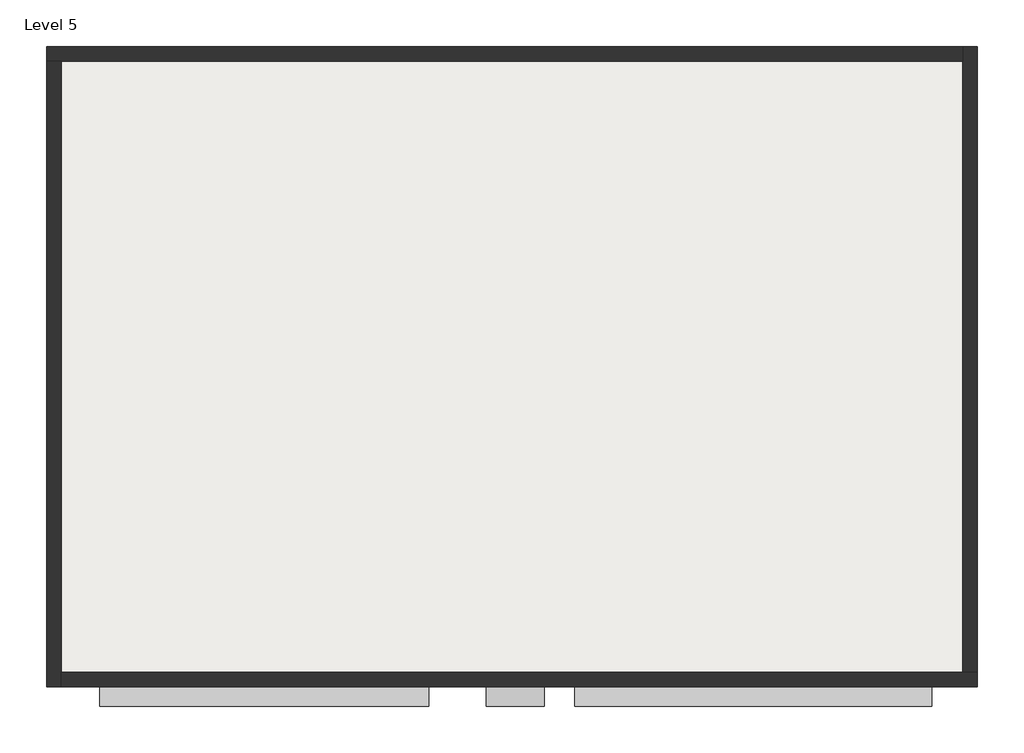
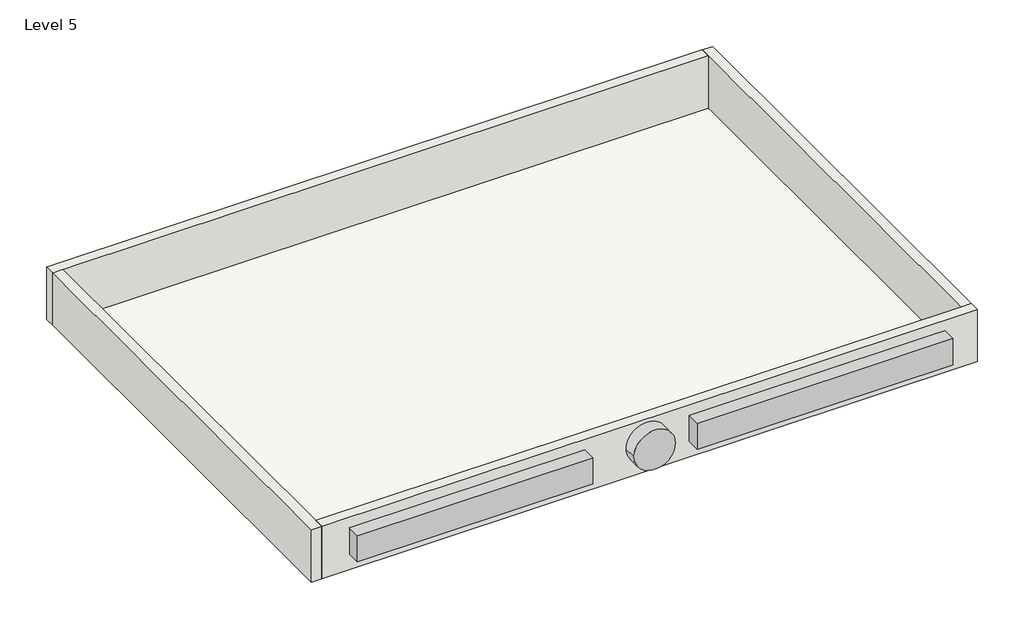
# One storey, incomplete: 4 walls, 1 proxy, 1 roof.
"""IFC4 building model written with IfcOpenShell, lengths in millimetres."""

from ifc_helpers import new_model, si_unit, frame, origin, place, context, project, spatial, polyline, outline, extrude, faceted_brep, transform, mapped, element, save
from components import generic_models_3_generic_models_3_f3c11b88

model = new_model("IFC4")

# Units and contexts
model_context = context("Model", 3, world=origin())
ifc_project = project(units=[si_unit("LENGTHUNIT", "METRE", prefix="MILLI")], contexts=[model_context])

# Site, building, storey
site = spatial("IfcSite", under=ifc_project)
building = spatial("IfcBuilding", under=site)
storey = spatial("IfcBuildingStorey", under=building, Name="Level 5", Elevation=9601.2)

# Proxy
placement = place(None, origin())
generic_models_3_generic_models_3_shape = generic_models_3_generic_models_3_f3c11b88(model_context)
element("IfcBuildingElementProxy", 1, Name="Generic Models 3 : Generic Models 3", ObjectType="Generic Models 3 : Generic Models 3", at=placement, inside=storey, context=model_context, shape_type="MappedRepresentation", body=[
    mapped(generic_models_3_generic_models_3_shape, transform((0.0, 0.0, 0.0), x_axis=(1.0, 0.0, 0.0), y_axis=(0.0, 1.0, 0.0), z_axis=(0.0, 0.0, 1.0))),
])

# Roof
element("IfcRoof", 2, ObjectType="Generic - 12\"", at=placement, inside=storey, context=model_context, shape_type="SweptSolid", body=[
    extrude(outline(polyline([(-8134.338363, 7846.5266064), (6077.748676, 7846.5266064), (6077.748676, -1794.1868249), (-8134.338363, -1794.1868249), (-8134.338363, 7846.5266064)])), frame((0.0, 0.0, 9448.8), z_axis=(0.0, 0.0, 1.0), x_axis=(1.0, 0.0, 0.0)), (0.0, 0.0, 1.0), 152.4),
])

# Walls
element("IfcWall", 3, ObjectType="WALL9\"", at=placement, inside=storey, context=model_context, shape_type="Brep", body=[
    faceted_brep([(-8362.938363, 7846.5266064, 9601.2), (-8134.338363, 7846.5266064, 9601.2), (6077.748676, 7846.5266064, 9601.2), (6077.748676, 7846.5266064, 10820.4), (-8134.338363, 7846.5266064, 10820.4), (-8362.938363, 7846.5266064, 10820.4), (-8362.938363, 8075.1266064, 9601.2), (-8362.938363, 8075.1266064, 10820.4), (6077.748676, 8075.1266064, 10820.4), (6077.748676, 8075.1266064, 9601.2)], [[[0, 1, 2, 3, 4, 5]], [[6, 7, 8, 9]], [[2, 1, 0, 6, 9]], [[5, 4, 3, 8, 7]], [[0, 5, 7, 6]], [[3, 2, 9, 8]]]),
])
element("IfcWall", 4, ObjectType="WALL9\"", at=placement, inside=storey, context=model_context, shape_type="Brep", body=[
    faceted_brep([(-8134.338363, -2022.7868249, 9601.2), (-8134.338363, -1794.1868249, 9601.2), (-8134.338363, 7846.5266064, 9601.2), (-8134.338363, 7846.5266064, 10820.4), (-8134.338363, -1794.1868249, 10820.4), (-8134.338363, -2022.7868249, 10820.4), (-8362.938363, -2022.7868249, 9601.2), (-8362.938363, -2022.7868249, 10820.4), (-8362.938363, 7846.5266064, 10820.4), (-8362.938363, 7846.5266064, 9601.2)], [[[0, 1, 2, 3, 4, 5]], [[6, 7, 8, 9]], [[2, 1, 0, 6, 9]], [[5, 4, 3, 8, 7]], [[0, 5, 7, 6]], [[3, 2, 9, 8]]]),
])
element("IfcWall", 5, ObjectType="WALL9\"", at=placement, inside=storey, context=model_context, shape_type="Brep", body=[
    faceted_brep([(6306.348676, -1794.1868249, 9601.2), (6077.748676, -1794.1868249, 9601.2), (-8134.338363, -1794.1868249, 9601.2), (-8134.338363, -1794.1868249, 10820.4), (6077.748676, -1794.1868249, 10820.4), (6306.348676, -1794.1868249, 10820.4), (6306.348676, -2022.7868249, 9601.2), (6306.348676, -2022.7868249, 10820.4), (-8134.338363, -2022.7868249, 10820.4), (-8134.338363, -2022.7868249, 9601.2)], [[[0, 1, 2, 3, 4, 5]], [[6, 7, 8, 9]], [[2, 1, 0, 6, 9]], [[5, 4, 3, 8, 7]], [[0, 5, 7, 6]], [[3, 2, 9, 8]]]),
])
element("IfcWall", 6, ObjectType="WALL9\"", at=placement, inside=storey, context=model_context, shape_type="Brep", body=[
    faceted_brep([(6077.748676, 8075.1266064, 9601.2), (6077.748676, 7846.5266064, 9601.2), (6077.748676, -1794.1868249, 9601.2), (6077.748676, -1794.1868249, 10820.4), (6077.748676, 7846.5266064, 10820.4), (6077.748676, 8075.1266064, 10820.4), (6306.348676, 8075.1266064, 9601.2), (6306.348676, 8075.1266064, 10820.4), (6306.348676, -1794.1868249, 10820.4), (6306.348676, -1794.1868249, 9601.2)], [[[0, 1, 2, 3, 4, 5]], [[6, 7, 8, 9]], [[2, 1, 0, 6, 9]], [[5, 4, 3, 8, 7]], [[0, 5, 7, 6]], [[3, 2, 9, 8]]]),
])

save(model, "model.ifc")

# Revit data of these elements
# Type "Generic - 12\""
#   Assembly Code = "B1020"
#   Layers, outside or top first: 0' - 6" no material (function 1)
# Type "WALL9\""
#   Assembly Code = "B2010"
#   Layers, outside or top first: 0' - 9" no material (function 1)
# Element 1 (IfcBuildingElementProxy, "Generic Models 3 : Generic Models 3")
#   Phase Created = New Construction
#   Materials on its faces: "sheets", "Parking Stripe"
# Element 2 (IfcRoof, "Generic - 12\"")
#   built-in parameter 1001705 = 31.5 (stored number, unit not read)
#   built-in parameter 1001701 = -0.5 (stored number, unit not read)
#   built-in parameter 1001710 = 33615
#   Phase Created = New Construction
#   Materials on its faces: "Default Roof"
# Elements 3, 4, 5, 6 (IfcWall, "WALL9\"")
#   Top Offset = 0' - 0"
#   Base Offset = 0' - 0"
#   Unconnected Height = 4' - 0"
#   wall height = 4' - 0"
#   Phase Created = New Construction
#   Base Constraint = Level 5
#   Materials on its faces: "Default Wall", "Cherry"
# Materials
#   "sheets": colour RGB 200 195 176, transparency 0, Cost = 0
#   "Parking Stripe": class "Paint", colour RGB 250 250 91, transparency 0, Cost = 0
#   "Default Roof": colour RGB 88 101 114, transparency 0, Cost = 0
#   "Default Wall": colour RGB 128 128 128, transparency 0, Cost = 0
#   "Cherry": class "Wood", colour RGB 226 177 128, transparency 0, Description = "Prunus Serotina", Cost = 0
